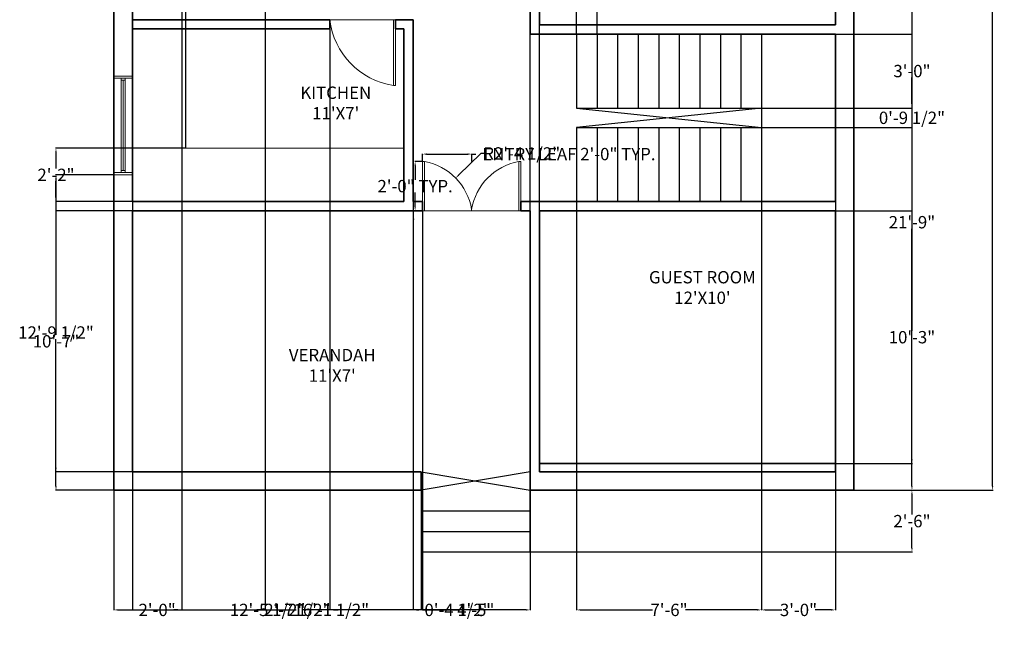
# Model space of a CAD drawing. Units: inches. Extents: x 897 to 1376, y 177 to 785.
# Tile 1 of 2: x 897 to 1376, y 177 to 473. Entities that reach past the tile are written whole.
import ezdxf

# ---------------------------------------------------------------- set-up
doc = ezdxf.new("R2010")
doc.units = ezdxf.units.IN
doc.header["$MEASUREMENT"] = 0
for name, color, linetype, lineweight in [('A-ANNO-DIMS', 2, 'Continuous', 13), ('A-AREA-IDEN', 7, 'Continuous', 18), ('A-DOOR', 3, 'Continuous', 18), ('A-FLOR-FIXT', 8, 'Continuous', 20), ('A-FLOR-STRS', 7, 'Continuous', 25), ('A-GLAZ', 4, 'Continuous', 18), ('A-WALL', 7, 'Continuous', 35)]:
    doc.layers.add(name, color=color, linetype=linetype, lineweight=lineweight)
doc.styles.get("Standard").update_dxf_attribs({"font": 'arial.ttf'})
doc.dimstyles.get("Standard").update_dxf_attribs({"dimtxt": 6, "dimasz": 2, "dimexe": 0.18, "dimexo": 0.0625, "dimgap": 0.09, "dimtad": 0, "dimtih": 1, "dimtoh": 1, "dimdec": 0, "dimzin": 0, "dimdsep": 46, "dimlunit": 4, "dimtxsty": 'Standard', "dimcen": 0.09, "dimadec": 0, "dimazin": 0, "dimtfac": 1, "dimtdec": 0, "dimtofl": 0, "dimtmove": 0, "dimatfit": 3, "dimfxl": 1, "dimtolj": 1, "dimtzin": 0, "dimarcsym": 0})

# ---------------------------------------------------------------- blocks, each defined once
blk = doc.blocks.new('RFEGTHYUJU')
for p, q in [((1141.26, 706.37), (1140.26, 706.37)), ((1140.26, 706.37), (1140.26, 674.37)), ((1141.26, 674.37), (1141.26, 706.37)), ((1141.26, 674.37), (1109.26, 674.37))]:
    blk.add_line(p, q)
blk.add_arc((1145.82, 669.96), 36.83, 98.6921, 173.1267)
blk = doc.blocks.new('*D6')
at = {"layer": 'A-ANNO-DIMS', "color": 0, "lineweight": -2, "transparency": 16777216}
for p, q in [((1302.82, 747.87), (1370.38, 747.87)), ((1370.2, 745.87), (1370.2, 498.97)), ((1370.2, 245.87), (1370.2, 492.76)), ((1302.82, 243.87), (1370.38, 243.87))]:
    blk.add_line(p, q, dxfattribs=at)
at = {"layer": 'A-ANNO-DIMS', "color": 0, "transparency": 16777216}
for points in [[(1369.87, 745.87), (1370.53, 745.87), (1370.2, 747.87)], [(1369.87, 245.87), (1370.53, 245.87), (1370.2, 243.87)]]:
    blk.add_solid(points, dxfattribs=at)
at = {"layer": 'Defpoints', "color": 0, "transparency": 16777216}
for p in [(1302.76, 747.87), (1302.76, 243.87), (1370.2, 243.87)]:
    blk.add_point(p, dxfattribs=at)
at = {"layer": 'A-ANNO-DIMS', "color": 0, "transparency": 16777216, "insert": (1370.2, 495.87), "char_height": 6, "attachment_point": 5}
blk.add_mtext("\\A1;42'", dxfattribs=at)
blk = doc.blocks.new('WIN-48IN-FRAMED')
for p, q in [((-24, 4.5), (-24, -4.5)), ((-23, 4.5), (-23, -4.5)), ((-23, 1), (23, 1)), ((-22, 1), (-22, -1)), ((22, 1), (22, -1)), ((23, 4.5), (23, -4.5)), ((24, 4.5), (24, -4.5)), ((-23, -1), (23, -1)), ((-22, 0), (22, 0))]:
    blk.add_line(p, q)
blk = doc.blocks.new('DOOR-LEAF-24IN')
for p, q in [((0, 0), (0, 24)), ((0, 24), (1, 24)), ((1, 24), (1, 0)), ((0, 0), (24, 0))]:
    blk.add_line(p, q)
blk.add_arc((-4.25, -4.05), 28.54, 9.4717, 79.4004)
blk = doc.blocks.new('*D14')
at = {"layer": 'A-ANNO-DIMS', "color": 0, "lineweight": -2, "transparency": 16777216}
for p, q in [((1092.86, 403.93), (1092.86, 407.65)), ((1094.86, 407.47), (1114.86, 407.47)), ((1116.86, 403.93), (1116.86, 407.65)), ((1116.86, 407.47), (1118.86, 407.47))]:
    blk.add_line(p, q, dxfattribs=at)
at = {"layer": 'A-ANNO-DIMS', "color": 0, "transparency": 16777216}
for points in [[(1094.86, 407.8), (1094.86, 407.13), (1092.86, 407.47)], [(1114.86, 407.8), (1114.86, 407.13), (1116.86, 407.47)]]:
    blk.add_solid(points, dxfattribs=at)
at = {"layer": 'Defpoints', "color": 0, "transparency": 16777216}
for p in [(1116.86, 407.47), (1092.86, 403.87), (1116.86, 403.87)]:
    blk.add_point(p, dxfattribs=at)
at = {"layer": 'A-ANNO-DIMS', "color": 0, "transparency": 16777216, "insert": (1164.09, 407.47), "char_height": 6, "attachment_point": 5}
blk.add_mtext('\\A1;ENTRY LEAF 2\'-0" TYP.', dxfattribs=at)
blk = doc.blocks.new('*D15')
at = {"layer": 'A-ANNO-DIMS', "color": 0, "lineweight": -2, "transparency": 16777216}
for p, q in [((1092.8, 403.87), (1089.08, 403.87)), ((1089.26, 401.87), (1089.26, 395.02)), ((1089.26, 381.87), (1089.26, 388.71)), ((1092.8, 379.87), (1089.08, 379.87))]:
    blk.add_line(p, q, dxfattribs=at)
at = {"layer": 'A-ANNO-DIMS', "color": 0, "transparency": 16777216}
for points in [[(1088.93, 401.87), (1089.59, 401.87), (1089.26, 403.87)], [(1088.93, 381.87), (1089.59, 381.87), (1089.26, 379.87)]]:
    blk.add_solid(points, dxfattribs=at)
at = {"layer": 'Defpoints', "color": 0, "transparency": 16777216}
for p in [(1089.26, 403.87), (1092.86, 403.87), (1092.86, 379.87)]:
    blk.add_point(p, dxfattribs=at)
at = {"layer": 'A-ANNO-DIMS', "color": 0, "transparency": 16777216, "insert": (1089.26, 391.87), "char_height": 6, "attachment_point": 5}
blk.add_mtext('\\A1;2\'-0" TYP.', dxfattribs=at)
blk = doc.blocks.new('*D16')
at = {"layer": 'A-ANNO-DIMS', "color": 0, "lineweight": -2, "transparency": 16777216}
for p, q in [((1145.32, 243.87), (1331.14, 243.87)), ((1330.96, 241.87), (1330.96, 232.02)), ((1330.96, 215.87), (1330.96, 225.71)), ((1145.32, 213.87), (1331.14, 213.87))]:
    blk.add_line(p, q, dxfattribs=at)
at = {"layer": 'A-ANNO-DIMS', "color": 0, "transparency": 16777216}
for points in [[(1330.63, 241.87), (1331.29, 241.87), (1330.96, 243.87)], [(1330.63, 215.87), (1331.29, 215.87), (1330.96, 213.87)]]:
    blk.add_solid(points, dxfattribs=at)
at = {"layer": 'Defpoints', "color": 0, "transparency": 16777216}
for p in [(1145.26, 243.87), (1330.96, 243.87), (1145.26, 213.87)]:
    blk.add_point(p, dxfattribs=at)
at = {"layer": 'A-ANNO-DIMS', "color": 0, "transparency": 16777216, "insert": (1330.96, 228.87), "char_height": 6, "attachment_point": 5}
blk.add_mtext('\\A1;2\'-6"', dxfattribs=at)
blk = doc.blocks.new('*D17')
at = {"layer": 'A-ANNO-DIMS', "color": 0, "lineweight": -2, "transparency": 16777216}
for p, q in [((1092.26, 213.8), (1092.26, 185.49)), ((1145.26, 213.8), (1145.26, 185.49)), ((1094.26, 185.67), (1110.57, 185.67)), ((1143.26, 185.67), (1126.94, 185.67))]:
    blk.add_line(p, q, dxfattribs=at)
at = {"layer": 'A-ANNO-DIMS', "color": 0, "transparency": 16777216}
for points in [[(1094.26, 186), (1094.26, 185.33), (1092.26, 185.67)], [(1143.26, 186), (1143.26, 185.33), (1145.26, 185.67)]]:
    blk.add_solid(points, dxfattribs=at)
at = {"layer": 'Defpoints', "color": 0, "transparency": 16777216}
for p in [(1092.26, 213.87), (1145.26, 213.87), (1145.26, 185.67)]:
    blk.add_point(p, dxfattribs=at)
at = {"layer": 'A-ANNO-DIMS', "color": 0, "transparency": 16777216, "insert": (1118.76, 185.67), "char_height": 6, "attachment_point": 5}
blk.add_mtext('\\A1;4\'-5"', dxfattribs=at)
blk = doc.blocks.new('*D18')
at = {"layer": 'A-ANNO-DIMS', "color": 0, "lineweight": -2, "transparency": 16777216}
for p, q in [((942.76, 243.8), (942.76, 185.49)), ((1092.26, 243.8), (1092.26, 185.49)), ((944.76, 185.67), (1000.41, 185.67)), ((1090.26, 185.67), (1034.61, 185.67))]:
    blk.add_line(p, q, dxfattribs=at)
at = {"layer": 'A-ANNO-DIMS', "color": 0, "transparency": 16777216}
for points in [[(944.76, 186), (944.76, 185.33), (942.76, 185.67)], [(1090.26, 186), (1090.26, 185.33), (1092.26, 185.67)]]:
    blk.add_solid(points, dxfattribs=at)
at = {"layer": 'Defpoints', "color": 0, "transparency": 16777216}
for p in [(942.76, 243.87), (1092.26, 243.87), (1092.26, 185.67)]:
    blk.add_point(p, dxfattribs=at)
at = {"layer": 'A-ANNO-DIMS', "color": 0, "transparency": 16777216, "insert": (1017.51, 185.67), "char_height": 6, "attachment_point": 5}
blk.add_mtext('\\A1;12\'-5 1/2"', dxfattribs=at)
blk = doc.blocks.new('*D22')
at = {"layer": 'A-ANNO-DIMS', "color": 0, "lineweight": -2, "transparency": 16777216}
for p, q in [((942.7, 397.43), (914.38, 397.43)), ((914.56, 395.43), (914.56, 323.84)), ((914.56, 245.87), (914.56, 317.46)), ((942.7, 243.87), (914.38, 243.87))]:
    blk.add_line(p, q, dxfattribs=at)
at = {"layer": 'A-ANNO-DIMS', "color": 0, "transparency": 16777216}
for points in [[(914.23, 395.43), (914.89, 395.43), (914.56, 397.43)], [(914.23, 245.87), (914.89, 245.87), (914.56, 243.87)]]:
    blk.add_solid(points, dxfattribs=at)
at = {"layer": 'Defpoints', "color": 0, "transparency": 16777216}
for p in [(914.56, 397.43), (942.76, 397.43), (942.76, 243.87)]:
    blk.add_point(p, dxfattribs=at)
at = {"layer": 'A-ANNO-DIMS', "color": 0, "transparency": 16777216, "insert": (914.56, 320.65), "char_height": 6, "attachment_point": 5}
blk.add_mtext('\\A1;12\'-9 1/2"', dxfattribs=at)
blk = doc.blocks.new('*D24')
at = {"layer": 'A-ANNO-DIMS', "color": 0, "lineweight": -2, "transparency": 16777216}
for p, q in [((1302.82, 504.76), (1331.14, 504.76)), ((1330.96, 502.76), (1330.96, 377.47)), ((1330.96, 245.87), (1330.96, 371.16)), ((1302.82, 243.87), (1331.14, 243.87))]:
    blk.add_line(p, q, dxfattribs=at)
at = {"layer": 'A-ANNO-DIMS', "color": 0, "transparency": 16777216}
for points in [[(1330.63, 502.76), (1331.29, 502.76), (1330.96, 504.76)], [(1330.63, 245.87), (1331.29, 245.87), (1330.96, 243.87)]]:
    blk.add_solid(points, dxfattribs=at)
at = {"layer": 'Defpoints', "color": 0, "transparency": 16777216}
for p in [(1302.76, 504.76), (1330.96, 504.76), (1302.76, 243.87)]:
    blk.add_point(p, dxfattribs=at)
at = {"layer": 'A-ANNO-DIMS', "color": 0, "transparency": 16777216, "insert": (1330.96, 374.32), "char_height": 6, "attachment_point": 5}
blk.add_mtext('\\A1;21\'-9"', dxfattribs=at)
blk = doc.blocks.new('*D25')
at = {"layer": 'A-ANNO-DIMS', "color": 0, "lineweight": -2, "transparency": 16777216}
for p, q in [((951.7, 379.87), (914.38, 379.87)), ((914.56, 377.87), (914.56, 319.52)), ((914.56, 254.87), (914.56, 313.21)), ((951.7, 252.87), (914.38, 252.87))]:
    blk.add_line(p, q, dxfattribs=at)
at = {"layer": 'A-ANNO-DIMS', "color": 0, "transparency": 16777216}
for points in [[(914.23, 377.87), (914.89, 377.87), (914.56, 379.87)], [(914.23, 254.87), (914.89, 254.87), (914.56, 252.87)]]:
    blk.add_solid(points, dxfattribs=at)
at = {"layer": 'Defpoints', "color": 0, "transparency": 16777216}
for p in [(914.56, 379.87), (951.76, 379.87), (951.76, 252.87)]:
    blk.add_point(p, dxfattribs=at)
at = {"layer": 'A-ANNO-DIMS', "color": 0, "transparency": 16777216, "insert": (914.56, 316.37), "char_height": 6, "attachment_point": 5}
blk.add_mtext('\\A1;10\'-7"', dxfattribs=at)
blk = doc.blocks.new('*D26')
at = {"layer": 'A-ANNO-DIMS', "color": 0, "lineweight": -2, "transparency": 16777216}
for p, q in [((1167.76, 384.3), (1167.76, 185.49)), ((1257.76, 384.3), (1257.76, 185.49)), ((1169.76, 185.67), (1204.72, 185.67)), ((1255.76, 185.67), (1220.8, 185.67))]:
    blk.add_line(p, q, dxfattribs=at)
at = {"layer": 'A-ANNO-DIMS', "color": 0, "transparency": 16777216}
for points in [[(1169.76, 186), (1169.76, 185.33), (1167.76, 185.67)], [(1255.76, 186), (1255.76, 185.33), (1257.76, 185.67)]]:
    blk.add_solid(points, dxfattribs=at)
at = {"layer": 'Defpoints', "color": 0, "transparency": 16777216}
for p in [(1167.76, 384.37), (1257.76, 384.37), (1257.76, 185.67)]:
    blk.add_point(p, dxfattribs=at)
at = {"layer": 'A-ANNO-DIMS', "color": 0, "transparency": 16777216, "insert": (1212.76, 185.67), "char_height": 6, "attachment_point": 5}
blk.add_mtext('\\A1;7\'-6"', dxfattribs=at)
blk = doc.blocks.new('*D27')
at = {"layer": 'A-ANNO-DIMS', "color": 0, "lineweight": -2, "transparency": 16777216}
for p, q in [((1257.76, 384.3), (1257.76, 185.49)), ((1293.76, 384.3), (1293.76, 185.49)), ((1259.76, 185.67), (1267.7, 185.67)), ((1291.76, 185.67), (1283.82, 185.67))]:
    blk.add_line(p, q, dxfattribs=at)
at = {"layer": 'A-ANNO-DIMS', "color": 0, "transparency": 16777216}
for points in [[(1259.76, 186), (1259.76, 185.33), (1257.76, 185.67)], [(1291.76, 186), (1291.76, 185.33), (1293.76, 185.67)]]:
    blk.add_solid(points, dxfattribs=at)
at = {"layer": 'Defpoints', "color": 0, "transparency": 16777216}
for p in [(1257.76, 384.37), (1293.76, 384.37), (1293.76, 185.67)]:
    blk.add_point(p, dxfattribs=at)
at = {"layer": 'A-ANNO-DIMS', "color": 0, "transparency": 16777216, "insert": (1275.76, 185.67), "char_height": 6, "attachment_point": 5}
blk.add_mtext('\\A1;3\'-0"', dxfattribs=at)
blk = doc.blocks.new('*D28')
at = {"layer": 'A-ANNO-DIMS', "color": 0, "lineweight": -2, "transparency": 16777216}
for p, q in [((1257.82, 465.87), (1331.14, 465.87)), ((1330.96, 463.87), (1330.96, 451.02)), ((1330.96, 431.87), (1330.96, 444.71)), ((1257.82, 429.87), (1331.14, 429.87))]:
    blk.add_line(p, q, dxfattribs=at)
at = {"layer": 'A-ANNO-DIMS', "color": 0, "transparency": 16777216}
for points in [[(1330.63, 463.87), (1331.29, 463.87), (1330.96, 465.87)], [(1330.63, 431.87), (1331.29, 431.87), (1330.96, 429.87)]]:
    blk.add_solid(points, dxfattribs=at)
at = {"layer": 'Defpoints', "color": 0, "transparency": 16777216}
for p in [(1257.76, 465.87), (1330.96, 465.87), (1257.76, 429.87)]:
    blk.add_point(p, dxfattribs=at)
at = {"layer": 'A-ANNO-DIMS', "color": 0, "transparency": 16777216, "insert": (1330.96, 447.87), "char_height": 6, "attachment_point": 5}
blk.add_mtext('\\A1;3\'-0"', dxfattribs=at)
blk = doc.blocks.new('*D29')
at = {"layer": 'A-ANNO-DIMS', "color": 0, "lineweight": -2, "transparency": 16777216}
for p, q in [((1145.26, 252.93), (1145.26, 776.25)), ((1147.26, 776.07), (1147.76, 776.07)), ((1149.76, 252.93), (1149.76, 776.25)), ((1149.76, 776.07), (1151.76, 776.07))]:
    blk.add_line(p, q, dxfattribs=at)
at = {"layer": 'A-ANNO-DIMS', "color": 0, "transparency": 16777216}
for points in [[(1147.26, 776.4), (1147.26, 775.73), (1145.26, 776.07)], [(1147.76, 776.4), (1147.76, 775.73), (1149.76, 776.07)]]:
    blk.add_solid(points, dxfattribs=at)
at = {"layer": 'Defpoints', "color": 0, "transparency": 16777216}
for p in [(1149.76, 776.07), (1145.26, 252.87), (1149.76, 252.87)]:
    blk.add_point(p, dxfattribs=at)
at = {"layer": 'A-ANNO-DIMS', "color": 0, "transparency": 16777216, "insert": (1166.81, 776.07), "char_height": 6, "attachment_point": 5}
blk.add_mtext('\\A1;0\'-4 1/2"', dxfattribs=at)
blk = doc.blocks.new('*D30')
at = {"layer": 'A-ANNO-DIMS', "color": 0, "lineweight": -2, "transparency": 16777216}
for p, q in [((951.76, 468.43), (951.76, 776.25)), ((953.76, 776.07), (956.64, 776.07)), ((975.76, 776.07), (972.87, 776.07)), ((977.76, 410.43), (977.76, 776.25))]:
    blk.add_line(p, q, dxfattribs=at)
at = {"layer": 'A-ANNO-DIMS', "color": 0, "transparency": 16777216}
for points in [[(953.76, 776.4), (953.76, 775.73), (951.76, 776.07)], [(975.76, 776.4), (975.76, 775.73), (977.76, 776.07)]]:
    blk.add_solid(points, dxfattribs=at)
at = {"layer": 'Defpoints', "color": 0, "transparency": 16777216}
for p in [(977.76, 776.07), (951.76, 468.37), (977.76, 410.37)]:
    blk.add_point(p, dxfattribs=at)
at = {"layer": 'A-ANNO-DIMS', "color": 0, "transparency": 16777216, "insert": (964.76, 776.07), "char_height": 6, "attachment_point": 5}
blk.add_mtext('\\A1;2\'-2"', dxfattribs=at)
blk = doc.blocks.new('*D31')
at = {"layer": 'A-ANNO-DIMS', "color": 0, "lineweight": -2, "transparency": 16777216}
for p, q in [((1330.96, 431.87), (1330.96, 433.87)), ((1257.82, 429.87), (1331.14, 429.87)), ((1257.82, 420.37), (1331.14, 420.37)), ((1330.96, 418.37), (1330.96, 416.37))]:
    blk.add_line(p, q, dxfattribs=at)
at = {"layer": 'A-ANNO-DIMS', "color": 0, "transparency": 16777216}
for points in [[(1330.63, 431.87), (1331.29, 431.87), (1330.96, 429.87)], [(1330.63, 418.37), (1331.29, 418.37), (1330.96, 420.37)]]:
    blk.add_solid(points, dxfattribs=at)
at = {"layer": 'Defpoints', "color": 0, "transparency": 16777216}
for p in [(1257.76, 429.87), (1330.96, 429.87), (1257.76, 420.37)]:
    blk.add_point(p, dxfattribs=at)
at = {"layer": 'A-ANNO-DIMS', "color": 0, "transparency": 16777216, "insert": (1330.96, 425.12), "char_height": 6, "attachment_point": 5}
blk.add_mtext('\\A1;0\'-9 1/2"', dxfattribs=at)
blk = doc.blocks.new('*D32')
at = {"layer": 'A-ANNO-DIMS', "color": 0, "lineweight": -2, "transparency": 16777216}
for p, q in [((1167.76, 465.93), (1167.76, 776.25)), ((1169.76, 776.07), (1175.76, 776.07)), ((1177.76, 465.93), (1177.76, 776.25)), ((1177.76, 776.07), (1179.76, 776.07))]:
    blk.add_line(p, q, dxfattribs=at)
at = {"layer": 'A-ANNO-DIMS', "color": 0, "transparency": 16777216}
for points in [[(1169.76, 776.4), (1169.76, 775.73), (1167.76, 776.07)], [(1175.76, 776.4), (1175.76, 775.73), (1177.76, 776.07)]]:
    blk.add_solid(points, dxfattribs=at)
at = {"layer": 'Defpoints', "color": 0, "transparency": 16777216}
for p in [(1177.76, 776.07), (1167.76, 465.87), (1177.76, 465.87)]:
    blk.add_point(p, dxfattribs=at)
at = {"layer": 'A-ANNO-DIMS', "color": 0, "transparency": 16777216, "insert": (1190.15, 776.07), "char_height": 6, "attachment_point": 5}
blk.add_mtext('\\A1;0\'-10"', dxfattribs=at)
blk = doc.blocks.new('*D33')
at = {"layer": 'A-ANNO-DIMS', "color": 0, "lineweight": -2, "transparency": 16777216}
for p, q in [((1088.26, 384.3), (1088.26, 185.49)), ((1092.86, 379.8), (1092.86, 185.49)), ((1090.26, 185.67), (1090.86, 185.67)), ((1092.86, 185.67), (1094.86, 185.67))]:
    blk.add_line(p, q, dxfattribs=at)
at = {"layer": 'A-ANNO-DIMS', "color": 0, "transparency": 16777216}
for points in [[(1090.26, 186), (1090.26, 185.33), (1088.26, 185.67)], [(1090.86, 186), (1090.86, 185.33), (1092.86, 185.67)]]:
    blk.add_solid(points, dxfattribs=at)
at = {"layer": 'Defpoints', "color": 0, "transparency": 16777216}
for p in [(1088.26, 384.37), (1092.86, 379.87), (1092.86, 185.67)]:
    blk.add_point(p, dxfattribs=at)
at = {"layer": 'A-ANNO-DIMS', "color": 0, "transparency": 16777216, "insert": (1109.91, 185.67), "char_height": 6, "attachment_point": 5}
blk.add_mtext('\\A1;0\'-4 1/2"', dxfattribs=at)
blk = doc.blocks.new('*D34')
at = {"layer": 'A-ANNO-DIMS', "color": 0, "lineweight": -2, "transparency": 16777216}
for p, q in [((951.76, 506.3), (951.76, 185.49)), ((975.76, 506.3), (975.76, 185.49)), ((953.76, 185.67), (955.64, 185.67)), ((973.76, 185.67), (971.87, 185.67))]:
    blk.add_line(p, q, dxfattribs=at)
at = {"layer": 'A-ANNO-DIMS', "color": 0, "transparency": 16777216}
for points in [[(953.76, 186), (953.76, 185.33), (951.76, 185.67)], [(973.76, 186), (973.76, 185.33), (975.76, 185.67)]]:
    blk.add_solid(points, dxfattribs=at)
at = {"layer": 'Defpoints', "color": 0, "transparency": 16777216}
for p in [(951.76, 506.37), (975.76, 506.37), (975.76, 185.67)]:
    blk.add_point(p, dxfattribs=at)
at = {"layer": 'A-ANNO-DIMS', "color": 0, "transparency": 16777216, "insert": (963.76, 185.67), "char_height": 6, "attachment_point": 5}
blk.add_mtext('\\A1;2\'-0"', dxfattribs=at)
blk = doc.blocks.new('*D35')
at = {"layer": 'A-ANNO-DIMS', "color": 0, "lineweight": -2, "transparency": 16777216}
for p, q in [((977.7, 410.37), (914.38, 410.37)), ((914.56, 408.37), (914.56, 400.47)), ((914.56, 386.37), (914.56, 394.26)), ((951.7, 384.37), (914.38, 384.37))]:
    blk.add_line(p, q, dxfattribs=at)
at = {"layer": 'A-ANNO-DIMS', "color": 0, "transparency": 16777216}
for points in [[(914.23, 408.37), (914.89, 408.37), (914.56, 410.37)], [(914.23, 386.37), (914.89, 386.37), (914.56, 384.37)]]:
    blk.add_solid(points, dxfattribs=at)
at = {"layer": 'Defpoints', "color": 0, "transparency": 16777216}
for p in [(977.76, 410.37), (914.56, 384.37), (951.76, 384.37)]:
    blk.add_point(p, dxfattribs=at)
at = {"layer": 'A-ANNO-DIMS', "color": 0, "transparency": 16777216, "insert": (914.56, 397.37), "char_height": 6, "attachment_point": 5}
blk.add_mtext('\\A1;2\'-2"', dxfattribs=at)
blk = doc.blocks.new('*D39')
at = {"layer": 'A-ANNO-DIMS', "color": 0, "lineweight": -2, "transparency": 16777216}
for p, q in [((951.76, 379.8), (951.76, 185.49)), ((1145.26, 379.8), (1145.26, 185.49)), ((953.76, 185.67), (1031.41, 185.67)), ((1143.26, 185.67), (1065.61, 185.67))]:
    blk.add_line(p, q, dxfattribs=at)
at = {"layer": 'A-ANNO-DIMS', "color": 0, "transparency": 16777216}
for points in [[(953.76, 186), (953.76, 185.33), (951.76, 185.67)], [(1143.26, 186), (1143.26, 185.33), (1145.26, 185.67)]]:
    blk.add_solid(points, dxfattribs=at)
at = {"layer": 'Defpoints', "color": 0, "transparency": 16777216}
for p in [(951.76, 379.87), (1145.26, 379.87), (1145.26, 185.67)]:
    blk.add_point(p, dxfattribs=at)
at = {"layer": 'A-ANNO-DIMS', "color": 0, "transparency": 16777216, "insert": (1048.51, 185.67), "char_height": 6, "attachment_point": 5}
blk.add_mtext('\\A1;16\'-1 1/2"', dxfattribs=at)
blk = doc.blocks.new('*D40')
at = {"layer": 'A-ANNO-DIMS', "color": 0, "lineweight": -2, "transparency": 16777216}
for p, q in [((1016.26, 501.8), (1016.26, 185.49)), ((1047.76, 472.8), (1047.76, 185.49)), ((1014.26, 185.67), (1012.26, 185.67)), ((1049.76, 185.67), (1051.76, 185.67))]:
    blk.add_line(p, q, dxfattribs=at)
at = {"layer": 'A-ANNO-DIMS', "color": 0, "transparency": 16777216}
for points in [[(1014.26, 186), (1014.26, 185.33), (1016.26, 185.67)], [(1049.76, 186), (1049.76, 185.33), (1047.76, 185.67)]]:
    blk.add_solid(points, dxfattribs=at)
at = {"layer": 'Defpoints', "color": 0, "transparency": 16777216}
for p in [(1016.26, 501.87), (1047.76, 472.87), (1016.26, 185.67)]:
    blk.add_point(p, dxfattribs=at)
at = {"layer": 'A-ANNO-DIMS', "color": 0, "transparency": 16777216, "insert": (1032.01, 185.67), "char_height": 6, "attachment_point": 5}
blk.add_mtext('\\A1;2\'-7 1/2"', dxfattribs=at)
blk = doc.blocks.new('*D41')
at = {"layer": 'A-ANNO-DIMS', "color": 0, "lineweight": -2, "transparency": 16777216}
for p, q in [((1293.82, 379.87), (1331.14, 379.87)), ((1330.96, 377.87), (1330.96, 321.52)), ((1330.96, 258.87), (1330.96, 315.21)), ((1293.82, 256.87), (1331.14, 256.87))]:
    blk.add_line(p, q, dxfattribs=at)
at = {"layer": 'A-ANNO-DIMS', "color": 0, "transparency": 16777216}
for points in [[(1330.63, 377.87), (1331.29, 377.87), (1330.96, 379.87)], [(1330.63, 258.87), (1331.29, 258.87), (1330.96, 256.87)]]:
    blk.add_solid(points, dxfattribs=at)
at = {"layer": 'Defpoints', "color": 0, "transparency": 16777216}
for p in [(1293.76, 379.87), (1330.96, 379.87), (1293.76, 256.87)]:
    blk.add_point(p, dxfattribs=at)
at = {"layer": 'A-ANNO-DIMS', "color": 0, "transparency": 16777216, "insert": (1330.96, 318.37), "char_height": 6, "attachment_point": 5}
blk.add_mtext('\\A1;10\'-3"', dxfattribs=at)
blk = doc.blocks.new('*D47')
at = {"layer": 'A-ANNO-DIMS', "color": 0, "lineweight": -2, "transparency": 16777216}
for p, q in [((1121.21, 407.78), (1110.42, 397.19)), ((1123.21, 407.78), (1121.21, 407.78)), ((1088.52, 375.81), (1088.7, 375.81)), ((1088.61, 375.72), (1088.61, 375.9))]:
    blk.add_line(p, q, dxfattribs=at)
at = {"layer": 'A-ANNO-DIMS', "color": 0, "transparency": 16777216}
blk.add_solid([(1110.18, 397.43), (1110.65, 396.96), (1108.99, 395.79)], dxfattribs=at)
at = {"layer": 'Defpoints', "color": 0, "transparency": 16777216}
for p in [(1108.99, 395.79), (1088.61, 375.81)]:
    blk.add_point(p, dxfattribs=at)
at = {"layer": 'A-ANNO-DIMS', "color": 0, "transparency": 16777216, "insert": (1141.14, 407.78), "char_height": 6, "attachment_point": 5}
blk.add_mtext('\\A1;R2\'-4 1/2"', dxfattribs=at)

msp = doc.modelspace()

# ---------------------------------------------------------------- linework, layer by layer
at = {"layer": 'A-DOOR'}
msp.add_line((1116.76, 380.51), (1116.76, 379.87), dxfattribs=at)
at = {"layer": 'A-FLOR-FIXT'}
for q in [(977.76, 468.37), (1083.76, 410.37)]:
    msp.add_line((977.76, 410.37), q, dxfattribs=at)
at = {"layer": 'A-FLOR-STRS'}
for p, q in [((1167.76, 465.87), (1167.76, 429.87)), ((1177.76, 465.87), (1177.76, 429.87)), ((1187.76, 465.87), (1187.76, 429.87)), ((1197.76, 465.87), (1197.76, 429.87)), ((1207.76, 465.87), (1207.76, 429.87)), ((1217.76, 465.87), (1217.76, 429.87)), ((1227.76, 465.87), (1227.76, 429.87)), ((1237.76, 465.87), (1237.76, 429.87)), ((1247.76, 465.87), (1247.76, 429.87)), ((1257.76, 465.87), (1257.76, 384.37)), ((1167.76, 429.87), (1257.76, 429.87)), ((1257.76, 429.87), (1167.76, 420.37)), ((1167.76, 429.87), (1257.76, 420.37)), ((1167.76, 420.37), (1257.76, 420.37)), ((1167.76, 420.37), (1167.76, 384.37)), ((1177.76, 420.37), (1177.76, 384.37)), ((1187.76, 420.37), (1187.76, 384.37)), ((1197.76, 420.37), (1197.76, 384.37)), ((1207.76, 420.37), (1207.76, 384.37)), ((1217.76, 420.37), (1217.76, 384.37)), ((1227.76, 420.37), (1227.76, 384.37)), ((1237.76, 420.37), (1237.76, 384.37)), ((1247.76, 420.37), (1247.76, 384.37)), ((1092.26, 252.87), (1145.26, 243.87)), ((1145.26, 252.87), (1092.26, 243.87))]:
    msp.add_line(p, q, dxfattribs=at)
for points in [[(1092.26, 243.87), (1092.26, 233.87), (1145.26, 233.87), (1145.26, 243.87)], [(1092.26, 233.87), (1092.26, 223.87), (1145.26, 223.87), (1145.26, 233.87)], [(1092.26, 223.87), (1092.26, 213.87), (1145.26, 213.87), (1145.26, 223.87)]]:
    msp.add_lwpolyline(points, dxfattribs=at)
at = {"layer": 'A-GLAZ'}
msp.add_line((942.76, 397.43), (951.76, 397.43), dxfattribs=at)
at = {"layer": 'A-WALL'}
for p, q in [((942.76, 243.87), (942.76, 747.87)), ((1302.76, 747.87), (1302.76, 243.87)), ((1293.76, 590.37), (1293.76, 470.37)), ((1145.26, 554.37), (1145.26, 465.87)), ((1149.76, 554.37), (1149.76, 470.37)), ((951.76, 472.87), (951.76, 501.87)), ((951.76, 472.87), (1047.76, 472.87)), ((1047.76, 468.37), (1047.76, 472.87)), ((1079.76, 468.37), (1079.76, 472.87)), ((1079.76, 472.87), (1088.26, 472.87)), ((1088.26, 384.37), (1088.26, 472.87)), ((1149.76, 470.37), (1293.76, 470.37)), ((951.76, 468.37), (1047.76, 468.37)), ((951.76, 384.37), (951.76, 468.37)), ((1079.76, 468.37), (1083.76, 468.37)), ((1083.76, 384.37), (1083.76, 468.37)), ((1145.26, 465.87), (1293.76, 465.87)), ((1293.76, 465.87), (1293.76, 384.37)), ((951.76, 384.37), (1083.76, 384.37)), ((1088.26, 384.37), (1092.86, 384.37)), ((1092.86, 379.87), (1092.86, 384.37)), ((1140.66, 384.37), (1140.66, 379.87)), ((1140.66, 384.37), (1293.76, 384.37)), ((1140.66, 379.87), (1140.66, 384.37)), ((951.76, 252.87), (951.76, 379.87)), ((951.76, 379.87), (1092.86, 379.87)), ((1140.66, 379.87), (1145.26, 379.87)), ((1145.26, 379.87), (1145.26, 243.87)), ((1149.76, 379.87), (1149.76, 252.87)), ((1149.76, 379.87), (1293.76, 379.87)), ((1293.76, 379.87), (1293.76, 252.87)), ((1293.76, 256.87), (1149.76, 256.87)), ((1092.26, 252.87), (951.76, 252.87)), ((1092.26, 252.87), (1092.26, 243.87)), ((1145.26, 243.87), (1145.26, 252.87)), ((1293.76, 252.87), (1149.76, 252.87)), ((1092.26, 243.87), (942.76, 243.87)), ((1302.76, 243.87), (1145.26, 243.87))]:
    msp.add_line(p, q, dxfattribs=at)

# ---------------------------------------------------------------- block references
at = {"layer": 'A-DOOR', "xscale": -1, "rotation": 180}
msp.add_blockref('RFEGTHYUJU', (-61.5, 1147.23), dxfattribs=at)
at = {"layer": 'A-DOOR'}
msp.add_blockref('DOOR-LEAF-24IN', (1092.86, 379.87), dxfattribs=at)
at = {"layer": 'A-DOOR', "extrusion": (0, 0, -1), "zscale": -1}
msp.add_blockref('DOOR-LEAF-24IN', (-1140.66, 379.87), dxfattribs=at)
at = {"layer": 'A-GLAZ', "rotation": 269.9999999999997}
msp.add_blockref('WIN-48IN-FRAMED', (947.26, 421.43), dxfattribs=at)

# ---------------------------------------------------------------- texts
at = {"layer": 'A-AREA-IDEN', "char_height": 6, "attachment_point": 1}
for s, width, insert in [("\\pxqc;KITCHEN^J11'X7'", 178.6551, (961.33, 440.33)), ("\\pxqc;GUEST ROOM^J12'X10'", 198.9149, (1129.56, 350.55)), ("\\pxqc;VERANDAH^J11'X7'", 172.5617, (962.65, 312.68))]:
    msp.add_mtext_dynamic_manual_height_columns(s, width=width, gutter_width=30, heights=[0], dxfattribs=dict(at, insert=insert))

# ---------------------------------------------------------------- dimensions: what is measured, and where the dimension line sits
at = {"layer": 'A-ANNO-DIMS'}
for base, p1, p2, picture, middle in [((1149.76, 776.07), (1145.26, 252.87), (1149.76, 252.87), '*D29', (1166.81, 776.07)), ((977.76, 776.07), (951.76, 468.37), (977.76, 410.37), '*D30', (964.76, 776.07)), ((1177.76, 776.07), (1167.76, 465.87), (1177.76, 465.87), '*D32', (1190.15, 776.07)), ((975.76, 185.67), (951.76, 506.37), (975.76, 506.37), '*D34', (963.76, 185.67)), ((1016.26, 185.67), (1047.76, 472.87), (1016.26, 501.87), '*D40', (1032.01, 185.67)), ((1092.86, 185.67), (1088.26, 384.37), (1092.86, 379.87), '*D33', (1109.91, 185.67)), ((1257.76, 185.67), (1167.76, 384.37), (1257.76, 384.37), '*D26', (1212.76, 185.67)), ((1293.76, 185.67), (1257.76, 384.37), (1293.76, 384.37), '*D27', (1275.76, 185.67)), ((1145.26, 185.67), (951.76, 379.87), (1145.26, 379.87), '*D39', (1048.51, 185.67)), ((1092.26, 185.67), (942.76, 243.87), (1092.26, 243.87), '*D18', (1017.51, 185.67)), ((1145.26, 185.67), (1092.26, 213.87), (1145.26, 213.87), '*D17', (1118.76, 185.67))]:
    dim = msp.add_linear_dim(base=base, p1=p1, p2=p2, dimstyle='Standard', override={"dimdec": 1, "dimlfac": 1, "dimrnd": 0, "dimzin": 1, "dimdsep": 46, "dimlunit": 4, "dimfrac": 2}, dxfattribs=at)
    dim.commit()
    dim.dimension.update_dxf_attribs({"geometry": picture, "text_midpoint": middle})
for base, p1, p2, override, picture, middle in [((1370.2, 243.87), (1302.76, 747.87), (1302.76, 243.87), {"dimclrd": 0, "dimclre": 0, "dimclrt": 0}, '*D6', (1370.2, 495.87)), ((1330.96, 504.76), (1302.76, 243.87), (1302.76, 504.76), {"dimdec": 1, "dimlfac": 1, "dimrnd": 0, "dimzin": 1, "dimdsep": 46, "dimlunit": 4, "dimfrac": 2}, '*D24', (1330.96, 374.32)), ((1330.96, 465.87), (1257.76, 429.87), (1257.76, 465.87), {"dimdec": 1, "dimlfac": 1, "dimrnd": 0, "dimzin": 1, "dimdsep": 46, "dimlunit": 4, "dimfrac": 2}, '*D28', (1330.96, 447.87)), ((1330.96, 429.87), (1257.76, 420.37), (1257.76, 429.87), {"dimdec": 1, "dimlfac": 1, "dimrnd": 0, "dimzin": 1, "dimdsep": 46, "dimlunit": 4, "dimfrac": 2}, '*D31', (1330.96, 425.12)), ((914.56, 384.37), (977.76, 410.37), (951.76, 384.37), {"dimdec": 1, "dimlfac": 1, "dimrnd": 0, "dimzin": 1, "dimdsep": 46, "dimlunit": 4, "dimfrac": 2}, '*D35', (914.56, 397.37)), ((914.56, 397.43), (942.76, 243.87), (942.76, 397.43), {"dimdec": 1, "dimlfac": 1, "dimrnd": 0, "dimzin": 1, "dimdsep": 46, "dimlunit": 4, "dimfrac": 2}, '*D22', (914.56, 320.65)), ((914.56, 379.87), (951.76, 252.87), (951.76, 379.87), {"dimdec": 1, "dimlfac": 1, "dimrnd": 0, "dimzin": 1, "dimdsep": 46, "dimlunit": 4, "dimfrac": 2}, '*D25', (914.56, 316.37)), ((1330.96, 379.87), (1293.76, 256.87), (1293.76, 379.87), {"dimdec": 1, "dimlfac": 1, "dimrnd": 0, "dimzin": 1, "dimdsep": 46, "dimlunit": 4, "dimfrac": 2}, '*D41', (1330.96, 318.37)), ((1330.96, 243.87), (1145.26, 213.87), (1145.26, 243.87), {"dimdec": 1, "dimlfac": 1, "dimrnd": 0, "dimzin": 1, "dimdsep": 46, "dimlunit": 4, "dimfrac": 2}, '*D16', (1330.96, 228.87))]:
    dim = msp.add_linear_dim(base=base, p1=p1, p2=p2, angle=90, dimstyle='Standard', override=override, dxfattribs=at)
    dim.commit()
    dim.dimension.update_dxf_attribs({"geometry": picture, "text_midpoint": middle})
dim = msp.add_linear_dim(base=(1116.86, 407.47), p1=(1092.86, 403.87), p2=(1116.86, 403.87), text='ENTRY LEAF <> TYP.', dimstyle='Standard', override={"dimdec": 1, "dimlfac": 1, "dimrnd": 0, "dimzin": 1, "dimdsep": 46, "dimlunit": 4, "dimfrac": 2}, dxfattribs=at)
dim.commit()
dim.dimension.update_dxf_attribs({"geometry": '*D14', "text_midpoint": (1164.09, 407.47)})
dim = msp.add_radius_dim(center=(1088.61, 375.81), mpoint=(1108.99, 395.79), dimstyle='Standard', override={"dimdec": 1, "dimlfac": 1, "dimrnd": 0, "dimzin": 1, "dimdsep": 46, "dimlunit": 4, "dimfrac": 2}, dxfattribs=at)
dim.commit()
dim.dimension.update_dxf_attribs({"geometry": '*D47', "text_midpoint": (1141.14, 407.78), "dimtype": 164})
dim = msp.add_linear_dim(base=(1089.26, 403.87), p1=(1092.86, 379.87), p2=(1092.86, 403.87), angle=90, text='<> TYP.', dimstyle='Standard', override={"dimdec": 1, "dimlfac": 1, "dimrnd": 0, "dimzin": 1, "dimdsep": 46, "dimlunit": 4, "dimfrac": 2}, dxfattribs=at)
dim.commit()
dim.dimension.update_dxf_attribs({"geometry": '*D15', "text_midpoint": (1089.26, 391.87)})

doc.saveas('drawing.dxf')
